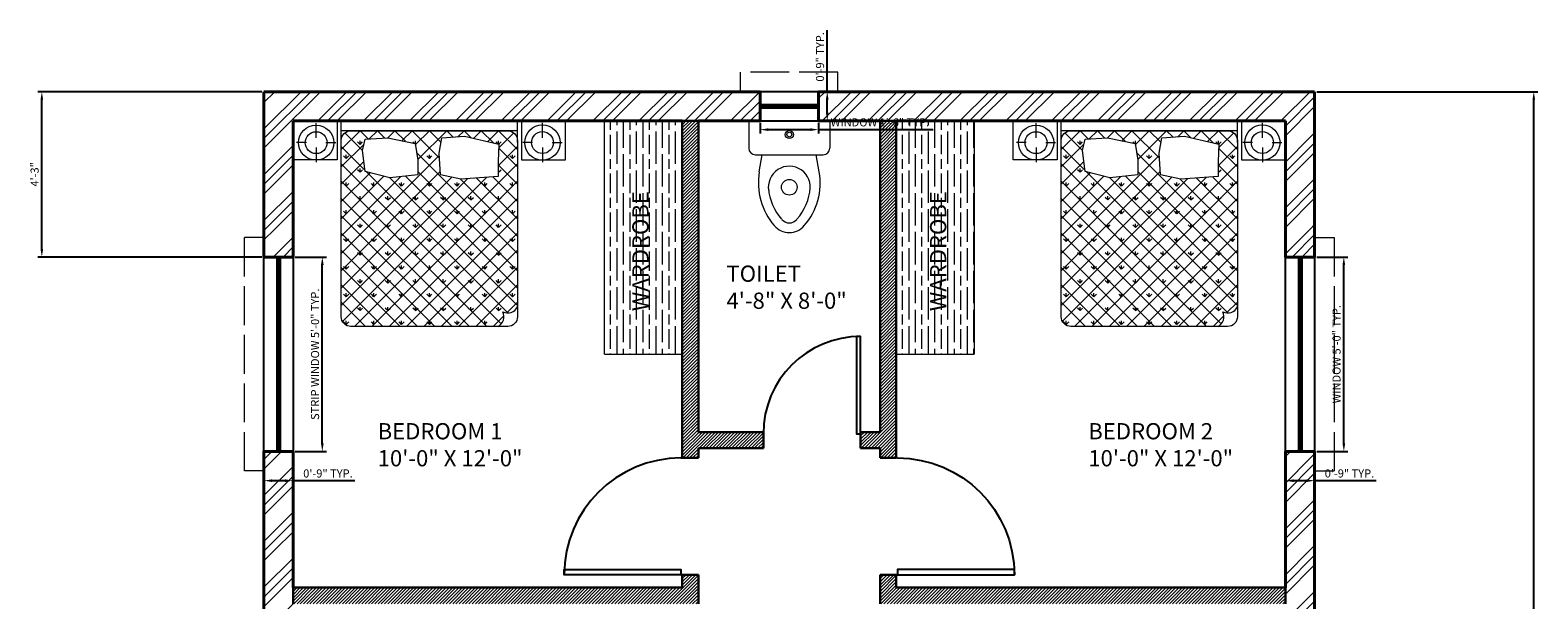
# Model space of a CAD drawing. Units: inches. Extents: x 2443635 to 2446153, y 1826255 to 1827341.
# Tile 5 of 16: x 2443635 to 2444100, y 1827149 to 1827324. Entities that reach past the tile are written whole.
import ezdxf

# ---------------------------------------------------------------- set-up
doc = ezdxf.new("R2010")
doc.units = ezdxf.units.IN
doc.linetypes.add('ACAD_ISO02W100', pattern=[15, 12, -3])
for name, color, linetype, lineweight in [('A-DIMS', 1, 'Continuous', 18), ('A-DOOR', 2, 'Continuous', 25), ('A-FLOR-CASE', 8, 'Continuous', 18), ('A-FLOR-CASE-PATT', 252, 'Continuous', 13), ('A-FLOR-FIXT', 9, 'Continuous', 18), ('A-FURN', 6, 'Continuous', 18), ('A-ROOM', 4, 'Continuous', 18), ('A-WALL-EXT', 7, 'Continuous', 40), ('A-WALL-INT', 9, 'Continuous', 30), ('A-WALL-OVHD', 7, 'ACAD_ISO02W100', 18), ('A-WALL-PATT', 8, 'Continuous', 13), ('A-WINDOW', 4, 'Continuous', 25)]:
    doc.layers.add(name, color=color, linetype=linetype, lineweight=lineweight)
doc.styles.get("Standard").update_dxf_attribs({"font": 'arial.ttf'})
doc.dimstyles.new('ISO-25', dxfattribs={"dimtxt": 2.5, "dimasz": 2.5, "dimexe": 1.25, "dimexo": 0.625, "dimtad": 1, "dimlunit": 4, "dimtxsty": 'Standard', "dimcen": 2.5, "dimadec": 0, "dimazin": 0, "dimtfac": 1, "dimtmove": 0, "dimatfit": 3, "dimfxl": 1, "dimarcsym": 0})

# ---------------------------------------------------------------- blocks, each defined once
blk = doc.blocks.new('*U2')
for p, q in [((0, 0), (0, -6)), ((40, 0), (40, -6))]:
    blk.add_line(p, q)
blk.add_lwpolyline([(0, 0), (0, 40), (1.75, 40), (1.75, 0)], close=True)
blk.add_arc((0, 0), 40, 0, 90)
blk = doc.blocks.new('*U3')
for p, q in [((0, 0), (0, -6)), ((-40, 0), (-40, -6))]:
    blk.add_line(p, q)
blk.add_lwpolyline([(0, 0), (0, 40), (-1.75, 40), (-1.75, 0)], close=True)
blk.add_arc((0, 0), 40, 90, 180)
blk = doc.blocks.new('*X6')
at = {"color": 0}
for p, q in [((0, 0), (0, 0)), ((-707, -141), (-734, -115)), ((-707, -141), (-707, -104)), ((-707, -141), (-681, -115)), ((-566, 0), (-566, 0)), ((-566, 0), (-566, 0)), ((-283, 0), (-283, 0)), ((-283, 0), (-283, 0)), ((-156, -126), (-168, -115)), ((-141, -141), (-142, -140)), ((-141, -141), (-141, -104)), ((-141, -141), (-115, -115)), ((120, -120), (115, -115)), ((283, 0), (283, 0)), ((566, 0), (566, 0)), ((699, -134), (681, -115)), ((707, -135), (707, -104)), ((710, -139), (734, -115)), ((-849, -283), (-875, -256)), ((-849, -283), (-849, -245)), ((-849, -283), (-822, -256)), ((0, -283), (-27, -256)), ((0, -283), (0, -245)), ((0, -283), (27, -256)), ((849, -283), (822, -256)), ((849, -283), (849, -245)), ((849, -283), (875, -256)), ((-707, -424), (-734, -398)), ((-707, -424), (-707, -387)), ((-707, -424), (-681, -398)), ((-116, -399), (-115, -398)), ((707, -424), (703, -420)), ((707, -424), (707, -387)), ((707, -424), (734, -398)), ((-849, -566), (-875, -539)), ((-849, -566), (-849, -528)), ((-849, -566), (-822, -539)), ((-566, -566), (-592, -539)), ((-566, -566), (-566, -528)), ((-566, -566), (-539, -539)), ((-283, -566), (-309, -539)), ((-283, -566), (-283, -528)), ((-283, -566), (-256, -539)), ((0, -566), (-27, -539)), ((0, -566), (0, -528)), ((0, -566), (27, -539)), ((283, -566), (256, -539)), ((283, -566), (283, -528)), ((283, -566), (309, -539)), ((566, -566), (539, -539)), ((566, -566), (566, -528)), ((566, -566), (592, -539)), ((849, -566), (822, -539)), ((849, -566), (849, -528)), ((849, -566), (875, -539)), ((-707, -707), (-734, -681)), ((-707, -707), (-707, -670)), ((-707, -707), (-681, -681)), ((-424, -707), (-451, -681)), ((-424, -707), (-424, -670)), ((-424, -707), (-398, -681)), ((-141, -707), (-168, -681)), ((-141, -707), (-141, -670)), ((-141, -707), (-115, -681)), ((141, -707), (115, -681)), ((141, -707), (141, -670)), ((141, -707), (168, -681)), ((424, -707), (398, -681)), ((424, -707), (424, -670)), ((424, -707), (451, -681)), ((707, -707), (681, -681)), ((707, -707), (707, -670)), ((707, -707), (734, -681)), ((-849, -849), (-875, -822)), ((-849, -849), (-849, -811)), ((-849, -849), (-822, -822)), ((-566, -849), (-592, -822)), ((-566, -849), (-566, -811)), ((-566, -849), (-539, -822)), ((-283, -849), (-309, -822)), ((-283, -849), (-283, -811)), ((-283, -849), (-256, -822)), ((0, -849), (-27, -822)), ((0, -849), (0, -811)), ((0, -849), (27, -822)), ((283, -849), (256, -822)), ((283, -849), (283, -811)), ((283, -849), (309, -822)), ((566, -849), (539, -822)), ((566, -849), (566, -811)), ((566, -849), (592, -822)), ((849, -849), (822, -822)), ((849, -849), (849, -811)), ((849, -849), (875, -822)), ((-707, -990), (-734, -963)), ((-707, -990), (-707, -952)), ((-707, -990), (-681, -963)), ((-424, -990), (-451, -963)), ((-424, -990), (-424, -952)), ((-424, -990), (-398, -963)), ((-141, -990), (-168, -963)), ((-141, -990), (-141, -952)), ((-141, -990), (-115, -963)), ((141, -990), (115, -963)), ((141, -990), (141, -952)), ((141, -990), (168, -963)), ((424, -990), (398, -963)), ((424, -990), (424, -952)), ((424, -990), (451, -963)), ((707, -990), (681, -963)), ((707, -990), (707, -952)), ((707, -990), (734, -963)), ((-849, -1131), (-875, -1105)), ((-849, -1131), (-849, -1094)), ((-849, -1131), (-822, -1105)), ((-566, -1131), (-592, -1105)), ((-566, -1131), (-566, -1094)), ((-566, -1131), (-539, -1105)), ((-283, -1131), (-309, -1105)), ((-283, -1131), (-283, -1094)), ((-283, -1131), (-256, -1105)), ((0, -1131), (-27, -1105)), ((0, -1131), (0, -1094)), ((0, -1131), (27, -1105)), ((283, -1131), (256, -1105)), ((283, -1131), (283, -1094)), ((283, -1131), (309, -1105)), ((566, -1131), (539, -1105)), ((566, -1131), (566, -1094)), ((566, -1131), (592, -1105)), ((849, -1131), (822, -1105)), ((849, -1131), (849, -1094)), ((849, -1131), (875, -1105)), ((-849, -1414), (-849, -1377)), ((-707, -1273), (-734, -1246)), ((-707, -1273), (-707, -1235)), ((-707, -1273), (-681, -1246)), ((-566, -1414), (-566, -1377)), ((-424, -1273), (-451, -1246)), ((-424, -1273), (-424, -1235)), ((-424, -1273), (-398, -1246)), ((-283, -1414), (-283, -1377)), ((-141, -1273), (-168, -1246)), ((-141, -1273), (-141, -1235)), ((-141, -1273), (-115, -1246)), ((0, -1414), (0, -1377)), ((141, -1273), (115, -1246)), ((141, -1273), (141, -1235)), ((141, -1273), (168, -1246)), ((283, -1414), (283, -1377)), ((424, -1273), (398, -1246)), ((424, -1273), (424, -1235)), ((424, -1273), (451, -1246)), ((566, -1414), (566, -1377)), ((707, -1273), (681, -1246)), ((707, -1273), (707, -1235)), ((707, -1273), (734, -1246)), ((849, -1414), (849, -1377)), ((-849, -1414), (-875, -1388)), ((-849, -1414), (-822, -1388)), ((-707, -1556), (-734, -1529)), ((-707, -1556), (-707, -1518)), ((-707, -1556), (-681, -1529)), ((-566, -1414), (-592, -1388)), ((-566, -1414), (-539, -1388)), ((-424, -1556), (-451, -1529)), ((-424, -1556), (-424, -1518)), ((-424, -1556), (-398, -1529)), ((-283, -1414), (-309, -1388)), ((-283, -1414), (-256, -1388)), ((-141, -1556), (-168, -1529)), ((-141, -1556), (-141, -1518)), ((-141, -1556), (-115, -1529)), ((0, -1414), (-27, -1388)), ((0, -1414), (27, -1388)), ((141, -1556), (115, -1529)), ((141, -1556), (141, -1518)), ((141, -1556), (168, -1529)), ((283, -1414), (256, -1388)), ((283, -1414), (309, -1388)), ((424, -1556), (398, -1529)), ((424, -1556), (424, -1518)), ((424, -1556), (451, -1529)), ((566, -1414), (539, -1388)), ((566, -1414), (592, -1388)), ((707, -1556), (681, -1529)), ((707, -1556), (707, -1518)), ((707, -1556), (734, -1529)), ((849, -1414), (822, -1388)), ((849, -1414), (875, -1388)), ((-849, -1697), (-875, -1671)), ((-849, -1697), (-849, -1660)), ((-849, -1697), (-822, -1671)), ((-566, -1697), (-592, -1671)), ((-566, -1697), (-566, -1660)), ((-566, -1697), (-539, -1671)), ((-283, -1697), (-309, -1671)), ((-283, -1697), (-283, -1660)), ((-283, -1697), (-256, -1671)), ((0, -1697), (-27, -1671)), ((0, -1697), (0, -1660)), ((0, -1697), (27, -1671)), ((283, -1697), (256, -1671)), ((283, -1697), (283, -1660)), ((283, -1697), (309, -1671)), ((566, -1697), (539, -1671)), ((566, -1697), (566, -1660)), ((566, -1697), (592, -1671)), ((849, -1697), (822, -1671)), ((849, -1697), (849, -1660)), ((849, -1697), (875, -1671)), ((-707, -1838), (-734, -1812)), ((-707, -1838), (-707, -1801)), ((-707, -1838), (-681, -1812)), ((-424, -1838), (-451, -1812)), ((-424, -1838), (-424, -1801)), ((-424, -1838), (-398, -1812)), ((-141, -1838), (-168, -1812)), ((-141, -1838), (-141, -1801)), ((-141, -1838), (-115, -1812)), ((141, -1838), (115, -1812)), ((141, -1838), (141, -1801)), ((141, -1838), (168, -1812)), ((424, -1838), (398, -1812)), ((424, -1838), (424, -1801)), ((424, -1838), (451, -1812)), ((707, -1838), (681, -1812)), ((707, -1838), (707, -1801)), ((707, -1838), (734, -1812)), ((-849, -1980), (-875, -1953)), ((-849, -1980), (-849, -1942)), ((-849, -1980), (-822, -1953)), ((-566, -1980), (-592, -1953)), ((-566, -1980), (-566, -1942)), ((-566, -1980), (-539, -1953)), ((-283, -1980), (-309, -1953)), ((-283, -1980), (-283, -1942)), ((-283, -1980), (-256, -1953)), ((0, -1980), (-27, -1953)), ((0, -1980), (0, -1942)), ((0, -1980), (27, -1953)), ((283, -1980), (256, -1953)), ((283, -1980), (283, -1942)), ((283, -1980), (309, -1953)), ((566, -1980), (539, -1953)), ((566, -1980), (566, -1942)), ((566, -1980), (592, -1953))]:
    blk.add_line(p, q, dxfattribs=at)
blk = doc.blocks.new('*X5')
at = {"color": 0}
for p, q in [((-900, -193), (-707, 0)), ((-623, -84), (-707, 0)), ((-614, -83), (-530, 0)), ((-457, -74), (-530, 0)), ((-425, -72), (-354, 0)), ((-245, -108), (-354, 0)), ((-278, -101), (-177, 0)), ((103, -280), (-177, 0)), ((-142, -142), (0, 0)), ((-117, -294), (177, 0)), ((120, -120), (0, 0)), ((241, -64), (177, 0)), ((292, -61), (354, 0)), ((426, -72), (354, 0)), ((452, -78), (530, 0)), ((654, -123), (530, 0)), ((596, -111), (707, 0)), ((900, -193), (707, 0)), ((-900, -370), (-667, -137)), ((-683, -201), (-862, -22)), ((708, -175), (862, -22)), ((-656, -405), (-900, -161)), ((-900, -1254), (101, -252)), ((900, -1254), (-128, -225)), ((703, -358), (900, -161)), ((900, -370), (708, -178)), ((-900, -546), (-668, -314)), ((735, -1973), (-900, -337)), ((-900, -1430), (112, -418)), ((-900, -723), (-605, -429)), ((-763, -2000), (900, -337)), ((801, -1862), (-641, -419)), ((900, -1430), (-116, -415)), ((900, -546), (703, -349)), ((-900, -900), (-465, -465)), ((-900, -1077), (-293, -470)), ((-900, -1607), (231, -476)), ((-900, -1784), (394, -489)), ((586, -2000), (-900, -514)), ((-888, -1948), (586, -475)), ((-586, -2000), (900, -514)), ((900, -1784), (-404, -480)), ((900, -1607), (-243, -465)), ((900, -1077), (317, -494)), ((900, -900), (483, -483)), ((900, -723), (647, -470)), ((409, -2000), (-900, -691)), ((-409, -2000), (900, -691)), ((232, -2000), (-900, -868)), ((-232, -2000), (900, -868)), ((55, -2000), (-900, -1045)), ((-55, -2000), (900, -1045)), ((-121, -2000), (-900, -1221)), ((121, -2000), (900, -1221)), ((-298, -2000), (-900, -1398)), ((298, -2000), (900, -1398)), ((-475, -2000), (-900, -1575)), ((475, -2000), (900, -1575)), ((-652, -2000), (-900, -1752)), ((790, -1861), (900, -1752)), ((-835, -1994), (-894, -1935)), ((652, -2000), (761, -1890))]:
    blk.add_line(p, q, dxfattribs=at)
blk = doc.blocks.new('A$C190D2546')
at = {"layer": 'A-FURN'}
for p, q in [((285, 1928), (285, 2078)), ((541, 2100), (2341, 2100)), ((541, 1881), (541, 2100)), ((2341, 1881), (2341, 2100)), ((2596, 1929), (2596, 2079)), ((185, 1878), (85, 1878)), ((385, 1878), (485, 1878)), ((2341, 2000), (541, 2000)), ((2496, 1879), (2396, 1879)), ((2696, 1879), (2796, 1879)), ((285, 1828), (285, 1678)), ((2596, 1829), (2596, 1679))]:
    blk.add_line(p, q, dxfattribs=at)
for points in [[(500, 2101), (500, 1701), (50, 1701), (50, 2101)], [(2382, 2101), (2382, 1701), (2832, 1701), (2832, 2101)], [(787, 1584), (758, 1799), (787, 1914), (1016, 1928), (1296, 1871), (1325, 1699), (1325, 1548), (1038, 1519)], [(1555, 1548), (1541, 1771), (1569, 1928), (1799, 1943), (2151, 1864), (2144, 1685), (2144, 1534), (1763, 1505)]]:
    blk.add_lwpolyline(points, close=True, dxfattribs=at)
blk.add_lwpolyline([(641, 2000), (2241, 2000, -0.414214), (2341, 1900), (2341, 100, -0.414214), (2241, 0), (641, 0, -0.414214), (541, 100), (541, 1900, -0.414214)], format="xyb", close=True, dxfattribs=at)
for centre, radius in [((285, 1878), 180), ((2596, 1879), 180), ((285, 1878), 112), ((2596, 1879), 112)]:
    blk.add_circle(centre, radius, dxfattribs=at)
for centre, start, end in [((2241, 250), 243.4349, 333.4349), ((2091, 100), 296.5651, 26.5651)]:
    blk.add_arc(centre, 112, start, end, dxfattribs=at)
for name in ['*X5', '*X6']:
    blk.add_blockref(name, (1441, 2000), dxfattribs=at)
blk = doc.blocks.new('WIN-18-PLAN')
at = {"transparency": 33554687}
for p, q in [((18, 9), (0, 9)), ((0, 9), (0, 0)), ((0, 5), (18, 5)), ((0.5, 5), (0.5, 4)), ((17.5, 4), (17.5, 5)), ((18, 0), (18, 9)), ((0, 4), (18, 4)), ((0.5, 4.5), (18, 4.5)), ((0, 0), (18, 0))]:
    blk.add_line(p, q, dxfattribs=at)
blk = doc.blocks.new('WIN-60-PLAN')
at = {"transparency": 33554687}
for p, q in [((0, 0), (0, 60)), ((0, 60), (9, 60)), ((4, 60), (4, 0)), ((4, 59.5), (5, 59.5)), ((4.5, 59.5), (4.5, 0.5)), ((5, 60), (5, 0)), ((9, 60), (9, 0)), ((5, 0.5), (4, 0.5)), ((9, 0), (0, 0))]:
    blk.add_line(p, q, dxfattribs=at)
blk = doc.blocks.new('WIN-60-STRIP-PLAN')
at = {"transparency": 33554687}
for p, q in [((0, 0), (0, 60)), ((4, 60), (4, 0)), ((4.5, 59.5), (4.5, 0.5)), ((5, 60), (5, 0)), ((9, 60), (9, 0))]:
    blk.add_line(p, q, dxfattribs=at)
blk = doc.blocks.new('WINDOW-HOOD-72-PLAN')
at = {"transparency": 33554687}
for p, q in [((0, 72), (6, 72)), ((6, 72), (6, 0)), ((0, 0), (6, 0))]:
    blk.add_line(p, q, dxfattribs=at)
blk = doc.blocks.new('WINDOW-HOOD-30-PLAN')
at = {"transparency": 33554687}
for p, q in [((30, 6), (0, 6)), ((0, 0), (0, 6)), ((30, 0), (30, 6))]:
    blk.add_line(p, q, dxfattribs=at)
blk = doc.blocks.new('*D80')
at = {"layer": 'A-DIMS', "color": 0, "lineweight": -2, "transparency": 16777216}
for p, q in [((2443860.09, 1827295.66), (2443860.09, 1827292.34)), ((2443862.59, 1827293.59), (2443875.59, 1827293.59)), ((2443878.09, 1827295.66), (2443878.09, 1827292.34)), ((2443878.09, 1827293.59), (2443913.48, 1827293.59))]:
    blk.add_line(p, q, dxfattribs=at)
at = {"layer": 'A-DIMS', "color": 0, "transparency": 16777216}
for points in [[(2443862.59, 1827294), (2443862.59, 1827293.17), (2443860.09, 1827293.59)], [(2443875.59, 1827294), (2443875.59, 1827293.17), (2443878.09, 1827293.59)]]:
    blk.add_solid(points, dxfattribs=at)
at = {"layer": 'Defpoints', "color": 0, "transparency": 16777216}
for p in [(2443860.09, 1827296.29), (2443878.09, 1827296.29), (2443878.09, 1827293.59)]:
    blk.add_point(p, dxfattribs=at)
at = {"layer": 'A-DIMS', "color": 0, "transparency": 16777216, "insert": (2443897.03, 1827295.51), "char_height": 2.5, "attachment_point": 5}
blk.add_mtext('WINDOW 1\'-6" TYP.', dxfattribs=at)
blk = doc.blocks.new('*D81')
at = {"layer": 'A-DIMS', "color": 0, "lineweight": -2, "transparency": 16777216}
for p, q in [((2443880.79, 1827305.29), (2443880.79, 1827324.28)), ((2443878.71, 1827305.29), (2443882.04, 1827305.29)), ((2443880.79, 1827298.79), (2443880.79, 1827302.79)), ((2443878.71, 1827296.29), (2443882.04, 1827296.29))]:
    blk.add_line(p, q, dxfattribs=at)
at = {"layer": 'A-DIMS', "color": 0, "transparency": 16777216}
for points in [[(2443880.37, 1827302.79), (2443881.21, 1827302.79), (2443880.79, 1827305.29)], [(2443880.37, 1827298.79), (2443881.21, 1827298.79), (2443880.79, 1827296.29)]]:
    blk.add_solid(points, dxfattribs=at)
at = {"layer": 'Defpoints', "color": 0, "transparency": 16777216}
for p in [(2443878.09, 1827305.29), (2443880.79, 1827305.29), (2443878.09, 1827296.29)]:
    blk.add_point(p, dxfattribs=at)
at = {"layer": 'A-DIMS', "color": 0, "transparency": 16777216, "insert": (2443878.89, 1827316.03), "char_height": 2.5, "attachment_point": 5, "rotation": 90}
blk.add_mtext('0\'-9" TYP.', dxfattribs=at)
blk = doc.blocks.new('*D82')
at = {"layer": 'A-DIMS', "color": 0, "lineweight": -2, "transparency": 16777216}
for p, q in [((2444031.71, 1827254.29), (2444041.34, 1827254.29)), ((2444040.09, 1827196.79), (2444040.09, 1827251.79)), ((2444031.71, 1827194.29), (2444041.34, 1827194.29))]:
    blk.add_line(p, q, dxfattribs=at)
at = {"layer": 'A-DIMS', "color": 0, "transparency": 16777216}
for points in [[(2444039.67, 1827251.79), (2444040.51, 1827251.79), (2444040.09, 1827254.29)], [(2444039.67, 1827196.79), (2444040.51, 1827196.79), (2444040.09, 1827194.29)]]:
    blk.add_solid(points, dxfattribs=at)
at = {"layer": 'Defpoints', "color": 0, "transparency": 16777216}
for p in [(2444031.09, 1827254.29), (2444040.09, 1827254.29), (2444031.09, 1827194.29)]:
    blk.add_point(p, dxfattribs=at)
at = {"layer": 'A-DIMS', "color": 0, "transparency": 16777216, "insert": (2444038.17, 1827224.29), "char_height": 2.5, "attachment_point": 5, "rotation": 90}
blk.add_mtext('WINDOW 5\'-0" TYP.', dxfattribs=at)
blk = doc.blocks.new('*D83')
at = {"layer": 'A-DIMS', "color": 0, "lineweight": -2, "transparency": 16777216}
for p, q in [((2444022.09, 1827193.66), (2444022.09, 1827184.04)), ((2444031.09, 1827193.66), (2444031.09, 1827184.04)), ((2444024.59, 1827185.29), (2444028.59, 1827185.29)), ((2444031.09, 1827185.29), (2444050.08, 1827185.29))]:
    blk.add_line(p, q, dxfattribs=at)
at = {"layer": 'A-DIMS', "color": 0, "transparency": 16777216}
for points in [[(2444024.59, 1827185.7), (2444024.59, 1827184.87), (2444022.09, 1827185.29)], [(2444028.59, 1827185.7), (2444028.59, 1827184.87), (2444031.09, 1827185.29)]]:
    blk.add_solid(points, dxfattribs=at)
at = {"layer": 'Defpoints', "color": 0, "transparency": 16777216}
for p in [(2444022.09, 1827194.29), (2444031.09, 1827194.29), (2444031.09, 1827185.29)]:
    blk.add_point(p, dxfattribs=at)
at = {"layer": 'A-DIMS', "color": 0, "transparency": 16777216, "insert": (2444041.83, 1827187.19), "char_height": 2.5, "attachment_point": 5}
blk.add_mtext('0\'-9" TYP.', dxfattribs=at)
blk = doc.blocks.new('*D84')
at = {"layer": 'A-DIMS', "color": 0, "lineweight": -2, "transparency": 16777216}
for p, q in [((2443716.71, 1827254.29), (2443726.34, 1827254.29)), ((2443725.09, 1827196.79), (2443725.09, 1827251.79)), ((2443716.71, 1827194.29), (2443726.34, 1827194.29))]:
    blk.add_line(p, q, dxfattribs=at)
at = {"layer": 'A-DIMS', "color": 0, "transparency": 16777216}
for points in [[(2443724.67, 1827251.79), (2443725.51, 1827251.79), (2443725.09, 1827254.29)], [(2443724.67, 1827196.79), (2443725.51, 1827196.79), (2443725.09, 1827194.29)]]:
    blk.add_solid(points, dxfattribs=at)
at = {"layer": 'Defpoints', "color": 0, "transparency": 16777216}
for p in [(2443716.09, 1827254.29), (2443725.09, 1827254.29), (2443716.09, 1827194.29)]:
    blk.add_point(p, dxfattribs=at)
at = {"layer": 'A-DIMS', "color": 0, "transparency": 16777216, "insert": (2443723.17, 1827224.29), "char_height": 2.5, "attachment_point": 5, "rotation": 90}
blk.add_mtext('STRIP WINDOW 5\'-0" TYP.', dxfattribs=at)
blk = doc.blocks.new('*D85')
at = {"layer": 'A-DIMS', "color": 0, "lineweight": -2, "transparency": 16777216}
for p, q in [((2443707.09, 1827193.66), (2443707.09, 1827184.04)), ((2443716.09, 1827193.66), (2443716.09, 1827184.04)), ((2443709.59, 1827185.29), (2443713.59, 1827185.29)), ((2443716.09, 1827185.29), (2443735.08, 1827185.29))]:
    blk.add_line(p, q, dxfattribs=at)
at = {"layer": 'A-DIMS', "color": 0, "transparency": 16777216}
for points in [[(2443709.59, 1827185.7), (2443709.59, 1827184.87), (2443707.09, 1827185.29)], [(2443713.59, 1827185.7), (2443713.59, 1827184.87), (2443716.09, 1827185.29)]]:
    blk.add_solid(points, dxfattribs=at)
at = {"layer": 'Defpoints', "color": 0, "transparency": 16777216}
for p in [(2443707.09, 1827194.29), (2443716.09, 1827194.29), (2443716.09, 1827185.29)]:
    blk.add_point(p, dxfattribs=at)
at = {"layer": 'A-DIMS', "color": 0, "transparency": 16777216, "insert": (2443726.83, 1827187.19), "char_height": 2.5, "attachment_point": 5}
blk.add_mtext('0\'-9" TYP.', dxfattribs=at)
blk = doc.blocks.new('*D91')
at = {"layer": 'A-DIMS', "color": 0, "lineweight": -2, "transparency": 16777216}
for p, q in [((2444031.71, 1827305.29), (2444099.91, 1827305.29)), ((2444098.66, 1826863.79), (2444098.66, 1827302.79)), ((2444031.71, 1826861.29), (2444099.91, 1826861.29))]:
    blk.add_line(p, q, dxfattribs=at)
at = {"layer": 'A-DIMS', "color": 0, "transparency": 16777216}
for points in [[(2444098.25, 1827302.79), (2444099.08, 1827302.79), (2444098.66, 1827305.29)], [(2444098.25, 1826863.79), (2444099.08, 1826863.79), (2444098.66, 1826861.29)]]:
    blk.add_solid(points, dxfattribs=at)
at = {"layer": 'Defpoints', "color": 0, "transparency": 16777216}
for p in [(2444031.09, 1827305.29), (2444098.66, 1827305.29), (2444031.09, 1826861.29)]:
    blk.add_point(p, dxfattribs=at)
at = {"layer": 'A-DIMS', "color": 0, "transparency": 16777216, "insert": (2444096.76, 1827083.29), "char_height": 2.5, "attachment_point": 5, "rotation": 90}
blk.add_mtext('37\'-0"', dxfattribs=at)
blk = doc.blocks.new('*D92')
at = {"layer": 'A-DIMS', "color": 0, "lineweight": -2, "transparency": 16777216}
for p, q in [((2443706.46, 1827305.29), (2443637.36, 1827305.29)), ((2443638.61, 1827256.79), (2443638.61, 1827302.79)), ((2443706.46, 1827254.29), (2443637.36, 1827254.29))]:
    blk.add_line(p, q, dxfattribs=at)
at = {"layer": 'A-DIMS', "color": 0, "transparency": 16777216}
for points in [[(2443638.19, 1827302.79), (2443639.02, 1827302.79), (2443638.61, 1827305.29)], [(2443638.19, 1827256.79), (2443639.02, 1827256.79), (2443638.61, 1827254.29)]]:
    blk.add_solid(points, dxfattribs=at)
at = {"layer": 'Defpoints', "color": 0, "transparency": 16777216}
for p in [(2443638.61, 1827305.29), (2443707.09, 1827305.29), (2443707.09, 1827254.29)]:
    blk.add_point(p, dxfattribs=at)
at = {"layer": 'A-DIMS', "color": 0, "transparency": 16777216, "insert": (2443636.7, 1827279.79), "char_height": 2.5, "attachment_point": 5, "rotation": 90}
blk.add_mtext('4\'-3"', dxfattribs=at)

msp = doc.modelspace()

# ---------------------------------------------------------------- hatches: boundary and pattern name
at = {"layer": 'A-FLOR-CASE-PATT'}
h = msp.add_hatch(dxfattribs=at)
h.set_pattern_fill('GOST_WOOD', color=256)
h.paths.add_polyline_path([(2443968.09, 1826966.288), (2443968.09, 1826990.288), (2443896.09, 1826990.288), (2443896.09, 1826966.288)])
h.paths.add_polyline_path([(2443902.09, 1827224.288), (2443926.09, 1827224.288), (2443926.09, 1827296.288), (2443902.09, 1827296.288)])
h.paths.add_polyline_path([(2443836.09, 1827296.288), (2443812.09, 1827296.288), (2443812.09, 1827224.288), (2443836.09, 1827224.288)])
at = {"layer": 'A-WALL-PATT'}
h = msp.add_hatch(dxfattribs=at)
h.set_pattern_fill('GOST_GROUND', color=256)
h.paths.add_polyline_path([(2443848.09, 1826870.288), (2443841.09, 1826870.288), (2443836.09, 1826870.288), (2443794.09, 1826870.288), (2443794.09, 1826861.288), (2443848.09, 1826861.288)])
h.paths.add_polyline_path([(2443935.09, 1826870.288), (2443896.09, 1826870.288), (2443891.09, 1826870.288), (2443884.09, 1826870.288), (2443884.09, 1826861.288), (2443935.09, 1826861.288)])
h.paths.add_polyline_path([(2444031.09, 1826999.288), (2444022.09, 1826999.288), (2444022.09, 1826995.288), (2444022.09, 1826990.288), (2444022.09, 1826870.288), (2443983.09, 1826870.288), (2443983.09, 1826861.288), (2444031.09, 1826861.288)])
h.paths.add_polyline_path([(2443758.09, 1826870.288), (2443716.09, 1826870.288), (2443716.09, 1826925.457, -0.0618154), (2443716.09, 1826925.788), (2443716.09, 1826948.288), (2443707.09, 1826948.288), (2443707.09, 1826861.288), (2443758.09, 1826861.288)])
h.paths.add_polyline_path([(2443716.09, 1827062.288), (2443716.09, 1827067.288), (2443716.09, 1827147.288), (2443716.09, 1827152.288), (2443716.09, 1827194.288), (2443707.09, 1827194.288), (2443707.09, 1826984.288), (2443716.09, 1826984.288)])
h.paths.add_polyline_path([(2443716.09, 1827296.288), (2443836.09, 1827296.288), (2443841.09, 1827296.288), (2443860.09, 1827296.288), (2443860.09, 1827305.288), (2443707.09, 1827305.288), (2443707.09, 1827254.288), (2443716.09, 1827254.288)])
h.paths.add_polyline_path([(2444031.09, 1827305.288), (2443878.09, 1827305.288), (2443878.09, 1827296.288), (2443881.588, 1827296.288), (2443897.09, 1827296.288), (2443902.09, 1827296.288), (2444022.09, 1827296.288), (2444022.09, 1827284.209), (2444022.09, 1827254.288), (2444031.09, 1827254.288)])
h.paths.add_polyline_path([(2444031.09, 1827194.288), (2444022.09, 1827194.288), (2444022.09, 1827152.288), (2444022.09, 1827147.288), (2444022.09, 1827113.953), (2444022.096, 1827113.948), (2444022.084, 1827080.628), (2444022.09, 1827047.288), (2444031.09, 1827047.288)])
h = msp.add_hatch(dxfattribs=at)
h.set_pattern_fill('JIS_WOOD', color=256)
h.paths.add_polyline_path([(2443841.09, 1827296.288), (2443836.09, 1827296.288), (2443836.09, 1827192.288), (2443841.09, 1827192.288), (2443841.09, 1827195.288), (2443861.09, 1827195.288), (2443861.09, 1827200.288), (2443841.09, 1827200.288)])
h.paths.add_polyline_path([(2443902.09, 1827296.288), (2443897.09, 1827296.288), (2443897.09, 1827200.288), (2443891.09, 1827200.288), (2443891.09, 1827195.288), (2443897.09, 1827195.288), (2443897.09, 1827192.288), (2443902.09, 1827192.288)])
h.paths.add_polyline_path([(2444022.09, 1827147.288), (2444022.09, 1827152.288), (2443902.09, 1827152.288), (2443902.09, 1827156.288), (2443897.09, 1827156.288), (2443897.09, 1827147.288)])
h.paths.add_polyline_path([(2443716.09, 1827152.288), (2443716.09, 1827147.288), (2443841.09, 1827147.288), (2443841.09, 1827156.288), (2443836.09, 1827156.288), (2443836.09, 1827152.288)])
h.paths.add_polyline_path([(2443836.09, 1827062.288), (2443836.09, 1827056.288), (2443841.09, 1827056.288), (2443841.09, 1827067.288), (2443716.09, 1827067.288), (2443716.09, 1827062.288)])
h.paths.add_polyline_path([(2443841.09, 1827020.288), (2443836.09, 1827020.288), (2443836.09, 1826870.288), (2443841.09, 1826870.288), (2443841.09, 1826966.288), (2443841.09, 1826971.288)])
h.paths.add_polyline_path([(2443896.09, 1826990.288), (2443980.09, 1826990.288), (2443980.09, 1826995.288), (2443891.09, 1826995.288), (2443891.09, 1826971.288), (2443891.09, 1826966.288), (2443891.09, 1826870.288), (2443896.09, 1826870.288)])

# ---------------------------------------------------------------- linework, layer by layer
at = {"layer": 'A-FLOR-CASE'}
for p, q in [((2443812.09, 1827224.288), (2443812.09, 1827296.288)), ((2443926.09, 1827296.288), (2443926.09, 1827224.288)), ((2443812.09, 1827224.288), (2443836.09, 1827224.288)), ((2443902.09, 1827224.288), (2443926.09, 1827224.288))]:
    msp.add_line(p, q, dxfattribs=at)
at = {"layer": 'A-FLOR-FIXT'}
for p, q in [((2443856.591, 1827296.288), (2443881.588, 1827296.288)), ((2443856.591, 1827296.288), (2443856.591, 1827287.865)), ((2443881.588, 1827296.288), (2443881.588, 1827287.865)), ((2443858.653, 1827285.803), (2443879.526, 1827285.803)), ((2443859.842, 1827280.555), (2443860.756, 1827285.795)), ((2443878.338, 1827280.555), (2443877.424, 1827285.795))]:
    msp.add_line(p, q, dxfattribs=at)
for centre, radius in [((2443869.09, 1827292.053), 1.25), ((2443869.09, 1827292.053), 0.75), ((2443869.095, 1827275.824), 2.41)]:
    msp.add_circle(centre, radius, dxfattribs=at)
for centre, radius, start, end in [((2443858.653, 1827287.865), 2.062, 180, 270), ((2443879.526, 1827287.865), 2.062, 270, 0), ((2443869.095, 1827275.824), 6.479, 347.37133, 190.68391), ((2443879.544, 1827277.119), 20, 170.10608, 221.06503), ((2443858.635, 1827277.119), 20, 318.93497, 9.89392), ((2443879.544, 1827277.119), 17, 185.68603, 221.06503), ((2443858.635, 1827277.119), 17, 318.93497, 355.06328), ((2443869.09, 1827267.803), 6, 219.57421, 270), ((2443869.09, 1827267.803), 3, 219.57421, 270), ((2443869.09, 1827267.803), 3, 270, 320.42579), ((2443869.09, 1827267.803), 6, 270, 320.42579)]:
    msp.add_arc(centre, radius, start, end, dxfattribs=at)
at = {"layer": 'A-WALL-EXT'}
for p, q in [((2443707.09, 1827305.288), (2443860.09, 1827305.288)), ((2443707.09, 1827254.288), (2443707.09, 1827305.288)), ((2443860.09, 1827305.288), (2443860.09, 1827296.288)), ((2443878.09, 1827305.288), (2443878.09, 1827296.288)), ((2443878.09, 1827305.288), (2444031.09, 1827305.288)), ((2444031.09, 1827305.288), (2444031.09, 1827254.288)), ((2443716.09, 1827296.288), (2443836.09, 1827296.288)), ((2443716.09, 1827254.288), (2443716.09, 1827296.288)), ((2443841.09, 1827296.288), (2443860.09, 1827296.288)), ((2443878.09, 1827296.288), (2443897.09, 1827296.288)), ((2443902.09, 1827296.288), (2444022.09, 1827296.288)), ((2444022.09, 1827296.288), (2444022.09, 1827254.288)), ((2443716.09, 1827254.288), (2443707.09, 1827254.288)), ((2444022.09, 1827254.288), (2444031.09, 1827254.288)), ((2443716.09, 1827194.288), (2443707.09, 1827194.288)), ((2443707.09, 1826984.288), (2443707.09, 1827194.288)), ((2443716.09, 1827152.288), (2443716.09, 1827194.288)), ((2444022.09, 1827194.288), (2444022.09, 1827152.288)), ((2444022.09, 1827194.288), (2444031.09, 1827194.288)), ((2444031.09, 1827194.288), (2444031.09, 1827047.288))]:
    msp.add_line(p, q, dxfattribs=at)
at = {"layer": 'A-WALL-INT'}
for p, q in [((2443836.09, 1827192.288), (2443836.09, 1827296.288)), ((2443836.09, 1827296.288), (2443841.09, 1827296.288)), ((2443841.09, 1827200.288), (2443841.09, 1827296.288)), ((2443897.09, 1827296.288), (2443897.09, 1827200.288)), ((2443897.09, 1827296.288), (2443902.09, 1827296.288)), ((2443902.09, 1827296.288), (2443902.09, 1827192.288)), ((2443841.09, 1827200.288), (2443861.09, 1827200.288)), ((2443861.09, 1827195.288), (2443861.09, 1827200.288)), ((2443891.09, 1827195.288), (2443891.09, 1827200.288)), ((2443891.09, 1827200.288), (2443897.09, 1827200.288)), ((2443841.09, 1827195.288), (2443861.09, 1827195.288)), ((2443841.09, 1827192.288), (2443841.09, 1827195.288)), ((2443891.09, 1827195.288), (2443897.09, 1827195.288)), ((2443897.09, 1827195.288), (2443897.09, 1827192.288)), ((2443836.09, 1827192.288), (2443841.09, 1827192.288)), ((2443902.09, 1827192.288), (2443897.09, 1827192.288)), ((2443716.09, 1827152.288), (2443836.09, 1827152.288)), ((2443716.09, 1827147.288), (2443716.09, 1827152.288)), ((2443836.09, 1827152.288), (2443836.09, 1827156.288)), ((2443836.09, 1827156.288), (2443841.09, 1827156.288)), ((2443841.09, 1827147.288), (2443841.09, 1827156.288)), ((2443902.09, 1827156.288), (2443897.09, 1827156.288)), ((2443897.09, 1827156.288), (2443897.09, 1827147.288)), ((2443902.09, 1827156.288), (2443902.09, 1827152.288)), ((2443902.09, 1827152.288), (2444022.09, 1827152.288)), ((2444022.09, 1827147.288), (2444022.09, 1827152.288))]:
    msp.add_line(p, q, dxfattribs=at)

# ---------------------------------------------------------------- block references
at = {"layer": 'A-DOOR', "xscale": 0.75, "yscale": 0.75, "zscale": 0.75}
msp.add_blockref('*U3', (2443891.09, 1827199.788), dxfattribs=at)
at = {"layer": 'A-DOOR', "yscale": 0.9, "zscale": 0.9}
for p, xscale, rotation in [((2443835.69, 1827156.288), 0.9, 90), ((2443902.49, 1827156.288), -0.9, 270)]:
    msp.add_blockref('*U2', p, dxfattribs=dict(at, xscale=xscale, rotation=rotation))
at = {"layer": 'A-FURN', "xscale": 0.0301964232523521, "yscale": 0.0301964232523521, "zscale": 0.0301964232523521}
for p in [(2443714.58, 1827232.854), (2443936.58, 1827232.854)]:
    msp.add_blockref('A$C190D2546', p, dxfattribs=at)
at = {"layer": 'A-WALL-OVHD', "transparency": 33554687}
for name, p in [('WINDOW-HOOD-30-PLAN', (2443854.09, 1827305.288)), ('WINDOW-HOOD-72-PLAN', (2444031.09, 1827188.288))]:
    msp.add_blockref(name, p, dxfattribs=at)
at = {"layer": 'A-WALL-OVHD', "transparency": 33554687, "rotation": 180}
msp.add_blockref('WINDOW-HOOD-72-PLAN', (2443707.09, 1827260.288), dxfattribs=at)
at = {"layer": 'A-WINDOW', "transparency": 33554687}
for name, p in [('WIN-18-PLAN', (2443860.09, 1827296.288)), ('WIN-60-STRIP-PLAN', (2443707.09, 1827194.288)), ('WIN-60-PLAN', (2444022.09, 1827194.288))]:
    msp.add_blockref(name, p, dxfattribs=at)

# ---------------------------------------------------------------- texts
at = {"layer": 'A-ROOM', "char_height": 5, "rotation": 90}
for insert, attachment_point in [((2443820.693, 1827237.573), 1), ((2443917.487, 1827237.573), 7)]:
    msp.add_mtext_dynamic_manual_height_columns('WARDROBE', width=52.37406, gutter_width=12.5, heights=[0], dxfattribs=dict(at, insert=insert, attachment_point=attachment_point))
at = {"layer": 'A-ROOM', "char_height": 5, "attachment_point": 1}
for s, insert in [('TOILET\\P4\'-8" X 8\'-0"', (2443849.712, 1827251.647)), ('BEDROOM 1\\P10\'-0" X 12\'-0"', (2443742.157, 1827203.042)), ('BEDROOM 2\\P10\'-0" X 12\'-0"', (2443961.283, 1827203.042))]:
    msp.add_mtext_dynamic_manual_height_columns(s, width=52.37406, gutter_width=12.5, heights=[0], dxfattribs=dict(at, insert=insert))

# ---------------------------------------------------------------- dimensions: what is measured, and where the dimension line sits
at = {"layer": 'A-DIMS', "transparency": 33554687}
for base, p1, p2, text, picture, middle in [((2443880.79, 1827305.288), (2443878.09, 1827296.288), (2443878.09, 1827305.288), '<> TYP.', '*D81', (2443878.888, 1827316.032)), ((2443725.09, 1827254.288), (2443716.09, 1827194.288), (2443716.09, 1827254.288), 'STRIP WINDOW <> TYP.', '*D84', (2443723.171, 1827224.288)), ((2444040.09, 1827254.288), (2444031.09, 1827194.288), (2444031.09, 1827254.288), 'WINDOW <> TYP.', '*D82', (2444038.171, 1827224.288))]:
    dim = msp.add_linear_dim(base=base, p1=p1, p2=p2, angle=90, text=text, dimstyle='ISO-25', override={"dimdec": 1, "dimlfac": 1, "dimrnd": 0, "dimzin": 1, "dimdsep": 46, "dimlunit": 4, "dimfrac": 2}, dxfattribs=at)
    dim.commit()
    dim.dimension.update_dxf_attribs({"geometry": picture, "text_midpoint": middle})
for base, p1, p2, picture, middle in [((2443638.607, 1827305.288), (2443707.09, 1827254.288), (2443707.09, 1827305.288), '*D92', (2443636.704, 1827279.788)), ((2444098.662, 1827305.288), (2444031.09, 1826861.288), (2444031.09, 1827305.288), '*D91', (2444096.76, 1827083.288))]:
    dim = msp.add_linear_dim(base=base, p1=p1, p2=p2, angle=90, dimstyle='ISO-25', override={"dimdec": 1, "dimlfac": 1, "dimrnd": 0, "dimzin": 1, "dimdsep": 46, "dimlunit": 4, "dimfrac": 2}, dxfattribs=at)
    dim.commit()
    dim.dimension.update_dxf_attribs({"geometry": picture, "text_midpoint": middle})
for base, p1, p2, text, picture, middle in [((2443878.09, 1827293.588), (2443860.09, 1827296.288), (2443878.09, 1827296.288), 'WINDOW <> TYP.', '*D80', (2443897.033, 1827295.506)), ((2443716.09, 1827185.288), (2443707.09, 1827194.288), (2443716.09, 1827194.288), '<> TYP.', '*D85', (2443726.834, 1827187.189)), ((2444031.09, 1827185.288), (2444022.09, 1827194.288), (2444031.09, 1827194.288), '<> TYP.', '*D83', (2444041.834, 1827187.189))]:
    dim = msp.add_linear_dim(base=base, p1=p1, p2=p2, text=text, dimstyle='ISO-25', override={"dimdec": 1, "dimlfac": 1, "dimrnd": 0, "dimzin": 1, "dimdsep": 46, "dimlunit": 4, "dimfrac": 2}, dxfattribs=at)
    dim.commit()
    dim.dimension.update_dxf_attribs({"geometry": picture, "text_midpoint": middle})

doc.saveas('drawing.dxf')
